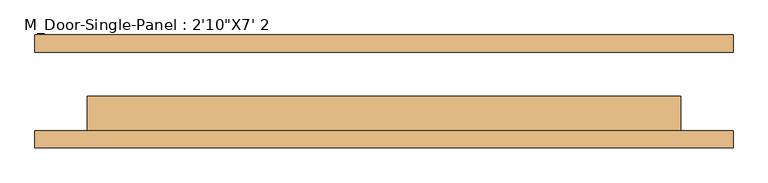
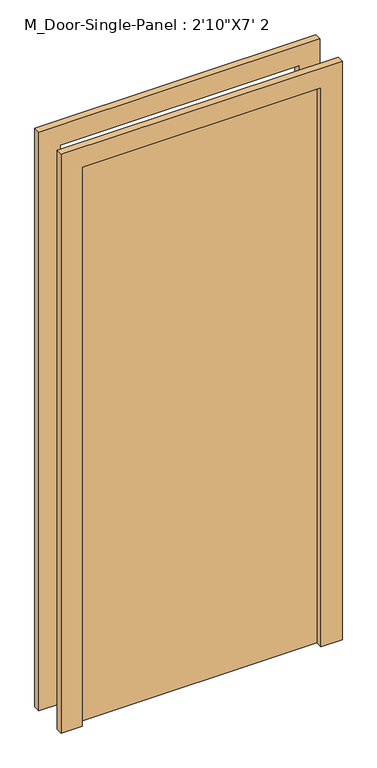
"""IFC4 building model written with IfcOpenShell, lengths in millimetres: door geometry."""

from ifc_helpers import new_model, si_unit, frame, origin, origin_with_axes, place, context, project, spatial, polyline, outline, extrude, source, transform, mapped, element, save


def door_85b31ab1(model_context):
    return source(origin(), model_context, "Body", "SweptSolid", [
        extrude(outline(polyline([(431.8, -7.15), (431.8, -57.15), (-431.8, -57.15), (-431.8, -7.15), (431.8, -7.15)])), origin_with_axes(), (0.0, 0.0, 1.0), 2133.6),
        extrude(outline(polyline([(2209.8, 508.0), (2209.8, -508.0), (0.0, -508.0), (0.0, -431.8), (2133.6, -431.8), (2133.6, 431.8), (0.0, 431.8), (0.0, 508.0), (2209.8, 508.0)])), frame((0.0, 57.15, 0.0), z_axis=(0.0, 1.0, 0.0), x_axis=(0.0, 0.0, 1.0)), (0.0, 0.0, 1.0), 25.0),
        extrude(outline(polyline([(2209.8, -508.0), (0.0, -508.0), (0.0, -431.8), (2133.6, -431.8), (2133.6, 431.8), (0.0, 431.8), (0.0, 508.0), (2209.8, 508.0), (2209.8, -508.0)])), frame((0.0, -82.15, 0.0), z_axis=(0.0, 1.0, 0.0), x_axis=(0.0, 0.0, 1.0)), (0.0, 0.0, 1.0), 25.0),
    ])


if __name__ == "__main__":
    model = new_model("IFC4")
    model_context = context("Model", 3, world=origin())
    ifc_project = project(units=[si_unit("LENGTHUNIT", "METRE", prefix="MILLI")], contexts=[model_context])
    site = spatial("IfcSite", under=ifc_project)
    building = spatial("IfcBuilding", under=site)
    placement = place(None, origin())
    door_shape = door_85b31ab1(model_context)
    element("IfcDoor", 1, ObjectType="M_Door-Single-Panel : 2'10\"X7' 2", at=placement, inside=building, context=model_context, shape_type="MappedRepresentation", body=[
        mapped(door_shape, transform((0.0, 0.0, 0.0), x_axis=(1.0, 0.0, 0.0), y_axis=(0.0, 1.0, 0.0), z_axis=(0.0, 0.0, 1.0))),
    ])
    save(model, "model.ifc")

# Revit data of these elements
# Type "M_Door-Single-Panel : 2'10\"X7' 2"
#   Type Mark = "10"
#   Construction Type Id = "DOOR"
#   Assembly Code = "C1020300"
#   Analytic Construction = "Wooden"
#   Thickness = 0' - 1.9685"
#   Thermal Resistance (R) = 2.5876 (h·ft²·°F)/BTU
#   Swing Angle [instance default] = 90.00°
#   Heat Transfer Coefficient (U) = 0.3865 BTU/(h·ft²·°F)
#   Height = 7' - 0"
#   Trim Projection Ext = 0' - 0.98425"
#   Trim Projection Int = 0' - 0.98425"
#   Trim Width = 0' - 3.14961"
#   Width = 2' - 10"
#   Define Thermal Properties by = 1
#   Panel Material = Wood - Birch - Solid Stained Light Low Gloss
#   Trim Material = Paint - Sienna
#   Visual Light Transmittance = 0
#   Solar Heat Gain Coefficient = 0
#   Function = (empty or 0)
#   Wall Closure = (empty or 0)
# Element 1 (IfcDoor, "M_Door-Single-Panel : 2'10\"X7' 2")
#   Materials on its faces: "Paint - Sienna", "Wood - Birch - Solid Stained Light Low Gloss"
# Materials
#   "Wood - Birch - Solid Stained Light Low Gloss": class "Wood", colour RGB 210 159 95, transparency 0, Cost = 0
#   "Paint - Sienna": colour RGB 118 70 51, transparency 0, Cost = 0
